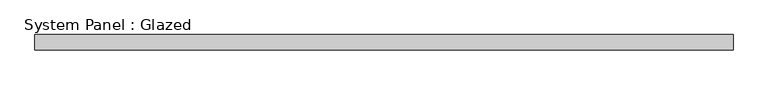
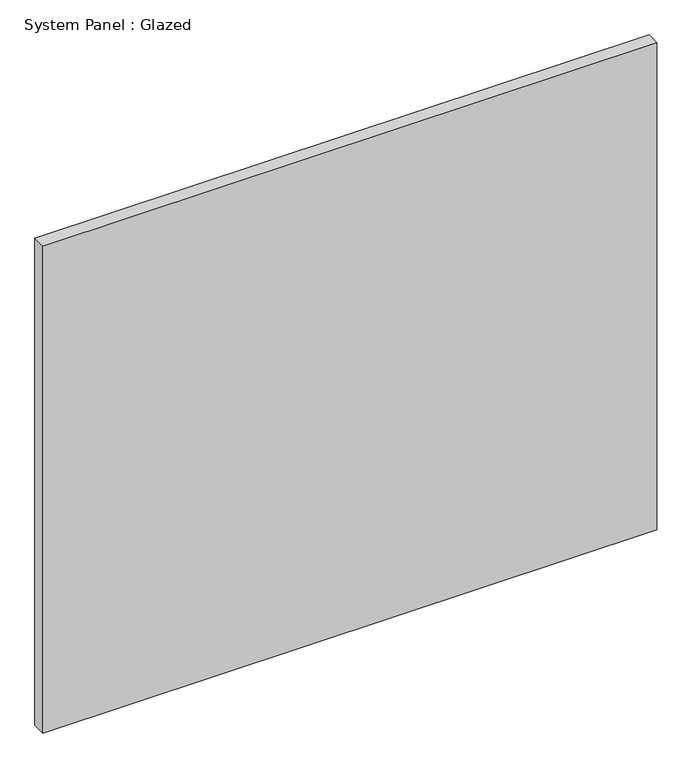
"""IFC4 building model written with IfcOpenShell, lengths in millimetres: plate geometry, System Panel : Glazed."""

from ifc_helpers import new_model, si_unit, origin, origin_with_axes, place, context, project, spatial, polyline, outline, extrude, source, transform, mapped, element, save


def system_panel_glazed_9bdbffb3(model_context):
    return source(origin(), model_context, "Body", "SweptSolid", [
        extrude(outline(polyline([(570.4416667, 19.05), (-570.4416667, 19.05), (-570.4416667, 44.45), (570.4416667, 44.45), (570.4416667, 19.05)])), origin_with_axes(), (0.0, 0.0, 1.0), 956.453622),
    ])


if __name__ == "__main__":
    model = new_model("IFC4")
    model_context = context("Model", 3, world=origin())
    ifc_project = project(units=[si_unit("LENGTHUNIT", "METRE", prefix="MILLI")], contexts=[model_context])
    site = spatial("IfcSite", under=ifc_project)
    building = spatial("IfcBuilding", under=site)
    placement = place(None, origin())
    system_panel_glazed_shape = system_panel_glazed_9bdbffb3(model_context)
    element("IfcPlate", 1, ObjectType="System Panel : Glazed", at=placement, inside=building, context=model_context, shape_type="MappedRepresentation", body=[
        mapped(system_panel_glazed_shape, transform((0.0, 0.0, 0.0), x_axis=(1.0, 0.0, 0.0), y_axis=(0.0, 1.0, 0.0), z_axis=(0.0, 0.0, 1.0))),
    ])
    save(model, "model.ifc")

# Revit data of these elements
# Type "System Panel : Glazed"
#   Construction Type Id = "GSP4R"
#   Analytic Construction = "1/8 in Pilkington single glazing"
#   Visual Light Transmittance = 0.9
#   Solar Heat Gain Coefficient = 0.86
#   Heat Transfer Coefficient (U) = 1.18115 BTU/(h·ft²·°F)
#   Define Thermal Properties by = 1
# Element 1 (IfcPlate, "System Panel : Glazed")
#   Materials on its faces: "Glass"
# Materials
#   "Glass": class "Glass", colour RGB 0 128 192, transparency 0.75, Description = "Soda Lime Glass", Cost = 0
